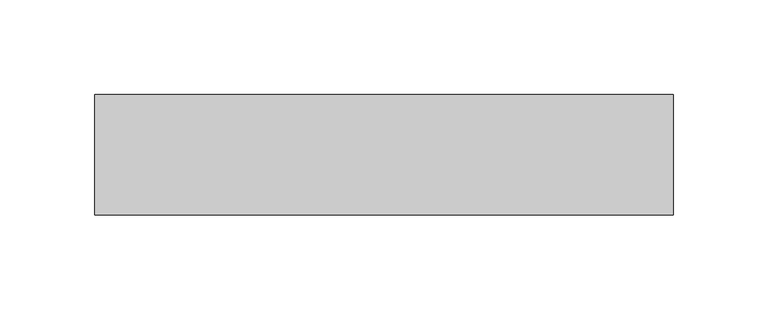
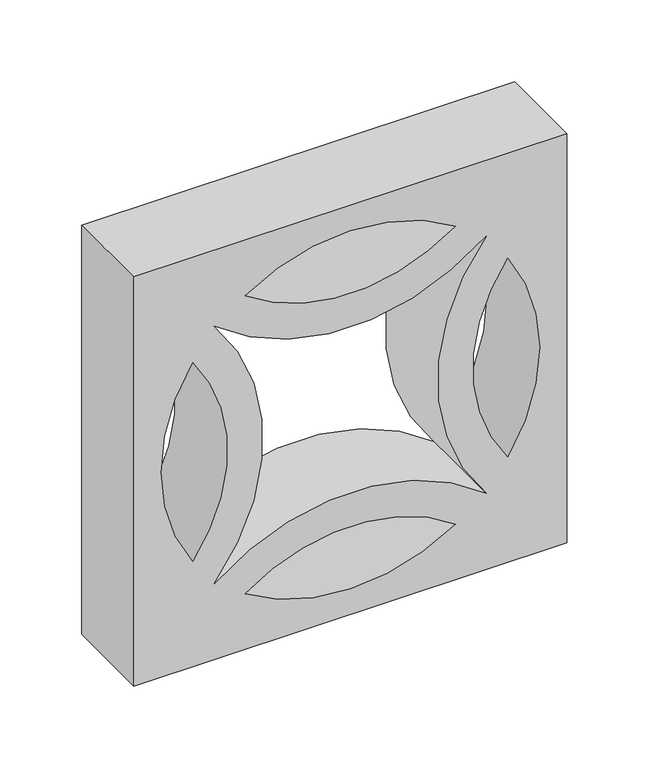
"""IFC4 building model written with IfcOpenShell, lengths in millimetres: plate geometry."""

from ifc_helpers import new_model, si_unit, point, frame, frame_2d, origin, place, context, project, spatial, polyline, circle_curve, trimmed, segment, composite_curve, outline, extrude, source, transform, mapped, element, save


def plate_14329628(model_context):
    return source(origin(), model_context, "Body", "SweptSolid", [
        extrude(outline(polyline([(304.8, -152.4), (0.0, -152.4), (0.0, 152.4), (304.8, 152.4), (304.8, -152.4)]), holes=[composite_curve([segment(trimmed(circle_curve(frame_2d((152.4, 0.0)), 133.35), [point((78.4367628, -110.9579291))], [point((226.3632372, -110.9579291))], True, "CARTESIAN"), True, "CONTINUOUS"), segment(trimmed(circle_curve(frame_2d((152.4, -211.3427385)), 124.690298), [point((226.3632372, -110.9579291))], [point((78.4367628, -110.9579291))], True, "CARTESIAN"), True, "CONTINUOUS")], self_intersect=False), composite_curve([segment(trimmed(circle_curve(frame_2d((152.4, 0.0)), 133.35), [point((263.3579291, -73.9632372))], [point((263.3579291, 73.9632372))], True, "CARTESIAN"), True, "CONTINUOUS"), segment(trimmed(circle_curve(frame_2d((363.7427385, 0.0)), 124.690298), [point((263.3579291, 73.9632372))], [point((263.3579291, -73.9632372))], True, "CARTESIAN"), True, "CONTINUOUS")], self_intersect=False), composite_curve([segment(trimmed(circle_curve(frame_2d((-58.9427385, 0.0)), 124.690298), [point((41.4420709, -73.9632372))], [point((41.4420709, 73.9632372))], True, "CARTESIAN"), True, "CONTINUOUS"), segment(trimmed(circle_curve(frame_2d((152.4, 0.0)), 133.35), [point((41.4420709, 73.9632372))], [point((41.4420709, -73.9632372))], True, "CARTESIAN"), True, "CONTINUOUS")], self_intersect=False), composite_curve([segment(trimmed(circle_curve(frame_2d((152.4, 0.0)), 133.35), [point((226.3632372, 110.9579291))], [point((78.4367628, 110.9579291))], True, "CARTESIAN"), True, "CONTINUOUS"), segment(trimmed(circle_curve(frame_2d((152.4, 211.3427385)), 124.690298), [point((78.4367628, 110.9579291))], [point((226.3632372, 110.9579291))], True, "CARTESIAN"), True, "CONTINUOUS")], self_intersect=False), composite_curve([segment(trimmed(circle_curve(frame_2d((363.7427385, 0.0)), 150.090298), [point((248.2169033, -95.8169033))], [point((248.2169033, 95.8169033))], False, "CARTESIAN"), True, "CONTINUOUS"), segment(trimmed(circle_curve(frame_2d((152.4, 211.3427385)), 150.090298), [point((248.2169033, 95.8169033))], [point((56.5830967, 95.8169033))], False, "CARTESIAN"), True, "CONTINUOUS"), segment(trimmed(circle_curve(frame_2d((-58.9427385, 0.0)), 150.090298), [point((56.5830967, 95.8169033))], [point((56.5830967, -95.8169033))], False, "CARTESIAN"), True, "CONTINUOUS"), segment(trimmed(circle_curve(frame_2d((152.4, -211.3427385)), 150.090298), [point((56.5830967, -95.8169033))], [point((248.2169033, -95.8169033))], False, "CARTESIAN"), True, "CONTINUOUS")], self_intersect=False)]), frame((0.0, -63.5, 0.0), z_axis=(0.0, 1.0, 0.0), x_axis=(0.0, 0.0, 1.0)), (0.0, 0.0, 1.0), 63.5),
    ])


if __name__ == "__main__":
    model = new_model("IFC4")
    model_context = context("Model", 3, world=origin())
    ifc_project = project(units=[si_unit("LENGTHUNIT", "METRE", prefix="MILLI")], contexts=[model_context])
    site = spatial("IfcSite", under=ifc_project)
    building = spatial("IfcBuilding", under=site)
    placement = place(None, origin())
    plate_shape = plate_14329628(model_context)
    element("IfcPlate", 1, at=placement, inside=building, context=model_context, shape_type="MappedRepresentation", body=[
        mapped(plate_shape, transform((0.0, 0.0, 0.0), x_axis=(1.0, 0.0, 0.0), y_axis=(0.0, 1.0, 0.0), z_axis=(0.0, 0.0, 1.0))),
    ])
    save(model, "model.ifc")
